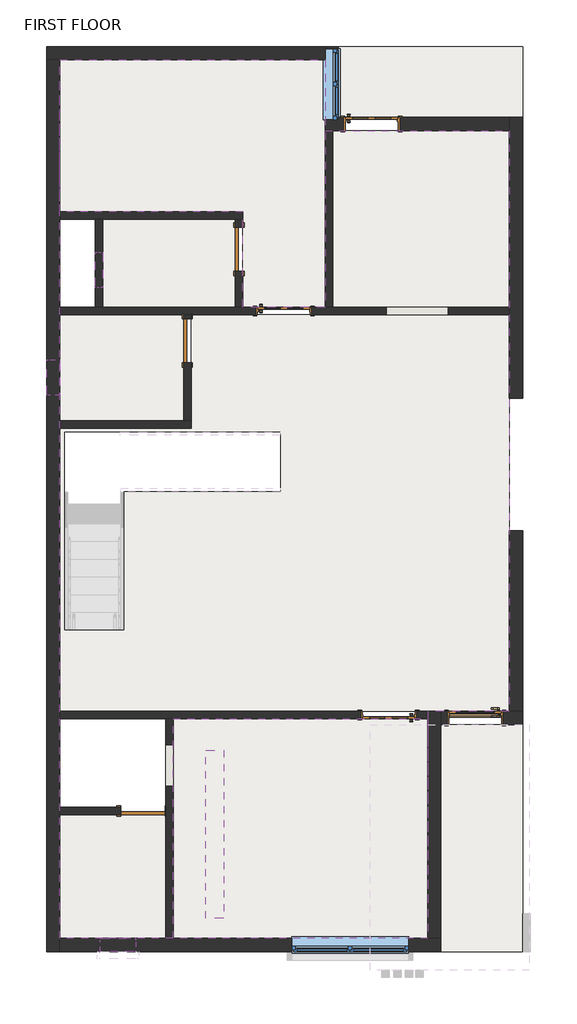
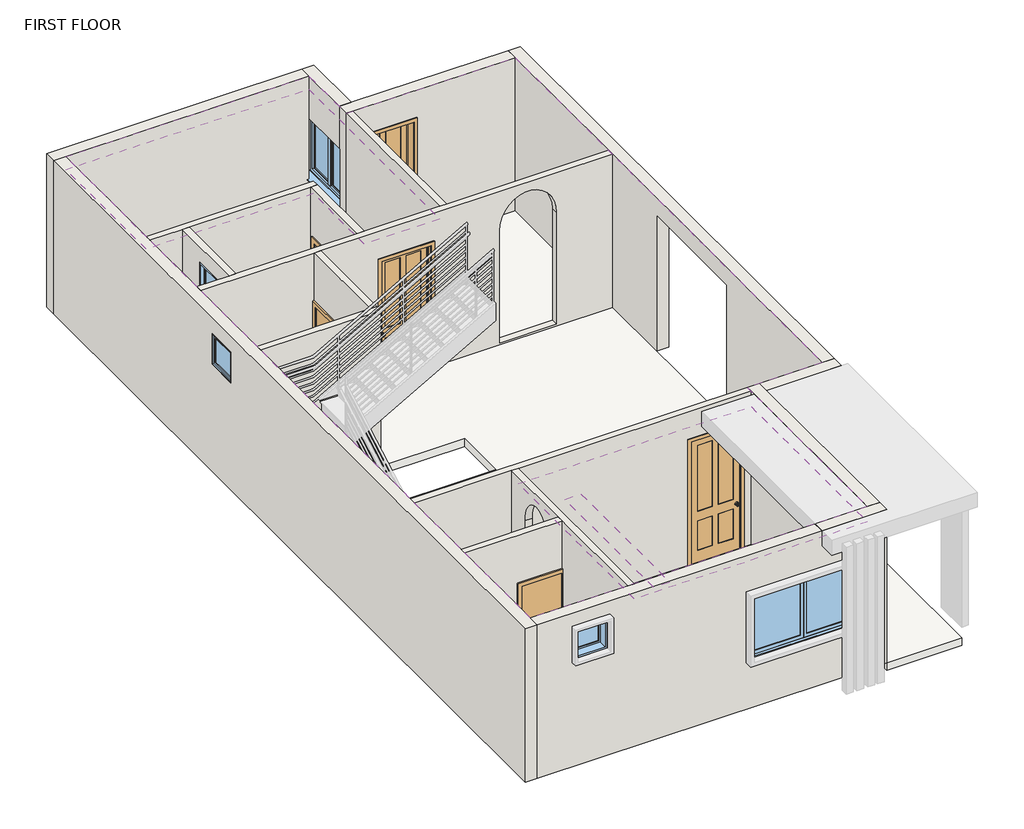
# One storey, part 1 of 3: 18 walls, 7 doors, 5 windows, 3 coverings, 3 slabs, 1 roof.
"""IFC4 building model written with IfcOpenShell, lengths in millimetres."""

from ifc_helpers import new_model, si_unit, point, frame, origin, place, context, project, spatial, polyline, ellipse_curve, trimmed, outline, extrude, faceted_brep, transform, mapped, element, save
from ifc_brep_helpers import plane_surface, extruded_surface, advanced_brep
from components import door_16625766, door_72f69035, door_4f3f9908, door_1fe7f57d, window_80340324, window_d757e824, w2_window_4_x_4_9dec5fc7, w2_window_6_x_4_7b90d420

model = new_model("IFC4")

# Units and contexts
model_context = context("Model", 3, world=origin())
ifc_project = project(units=[si_unit("LENGTHUNIT", "METRE", prefix="MILLI")], contexts=[model_context])

# Site, building, storey
site = spatial("IfcSite", under=ifc_project)
building = spatial("IfcBuilding", under=site)
storey = spatial("IfcBuildingStorey", under=building, Name="FIRST FLOOR", Elevation=3352.8)

# Coverings
placement = place(None, origin())
element("IfcCovering", 1, at=placement, inside=storey, context=model_context, shape_type="SweptSolid", body=[
    extrude(outline(polyline([(-4259.325552, -303.3614843), (-4259.325552, -3198.9614843), (-4564.125552, -3198.9614843), (-4564.125552, -303.3614843), (-4259.325552, -303.3614843)])), frame((0.0, 0.0, 5918.2), z_axis=(0.0, 0.0, 1.0), x_axis=(1.0, 0.0, 0.0)), (0.0, 0.0, 1.0), 41.275),
    extrude(outline(polyline([(-3649.725552, -303.3614843), (-3649.725552, -3198.9614843), (-3954.525552, -3198.9614843), (-3954.525552, -303.3614843), (-3649.725552, -303.3614843)])), frame((0.0, 0.0, 5918.2), z_axis=(0.0, 0.0, 1.0), x_axis=(1.0, 0.0, 0.0)), (0.0, 0.0, 1.0), 41.275),
    extrude(outline(polyline([(-3065.525552, -303.3614843), (-3065.525552, -3198.9614843), (-3370.325552, -3198.9614843), (-3370.325552, -303.3614843), (-3065.525552, -303.3614843)])), frame((0.0, 0.0, 5918.2), z_axis=(0.0, 0.0, 1.0), x_axis=(1.0, 0.0, 0.0)), (0.0, 0.0, 1.0), 41.275),
    extrude(outline(polyline([(-2455.925552, -303.3614843), (-2455.925552, -3198.9614843), (-2760.725552, -3198.9614843), (-2760.725552, -303.3614843), (-2455.925552, -303.3614843)])), frame((0.0, 0.0, 5918.2), z_axis=(0.0, 0.0, 1.0), x_axis=(1.0, 0.0, 0.0)), (0.0, 0.0, 1.0), 41.275),
    extrude(outline(polyline([(-1846.325552, -303.3614843), (-1846.325552, -3198.9614843), (-2151.125552, -3198.9614843), (-2151.125552, -303.3614843), (-1846.325552, -303.3614843)])), frame((0.0, 0.0, 5918.2), z_axis=(0.0, 0.0, 1.0), x_axis=(1.0, 0.0, 0.0)), (0.0, 0.0, 1.0), 41.275),
    extrude(outline(polyline([(-1236.725552, -303.3614843), (-1236.725552, -3198.9614843), (-1541.525552, -3198.9614843), (-1541.525552, -303.3614843), (-1236.725552, -303.3614843)])), frame((0.0, 0.0, 5918.2), z_axis=(0.0, 0.0, 1.0), x_axis=(1.0, 0.0, 0.0)), (0.0, 0.0, 1.0), 41.275),
])
element("IfcCovering", 2, at=placement, inside=storey, context=model_context, shape_type="SweptSolid", body=[
    extrude(outline(polyline([(-7080.273248, 8978.3133697), (-7080.273248, 11594.5133697), (-2508.273248, 11594.5133697), (-2508.273248, 7327.3133697), (-3930.673248, 7327.3133697), (-3930.673248, 8978.3133697), (-7080.273248, 8978.3133697)]), holes=[polyline([(-6775.473248, 11289.7133697), (-6775.473248, 9283.1133697), (-3625.873248, 9283.1133697), (-3625.873248, 7632.1133697), (-2813.073248, 7632.1133697), (-2813.073248, 11289.7133697), (-6775.473248, 11289.7133697)])]), frame((0.0, 0.0, 6146.8), z_axis=(0.0, 0.0, 1.0), x_axis=(1.0, 0.0, 0.0)), (0.0, 0.0, 1.0), 107.95),
    extrude(outline(polyline([(-3422.673248, 10680.1133697), (-3422.673248, 9892.7133697), (-6165.873248, 9892.7133697), (-6165.873248, 10680.1133697), (-3422.673248, 10680.1133697)])), frame((0.0, 0.0, 6146.8), z_axis=(0.0, 0.0, 1.0), x_axis=(1.0, 0.0, 0.0)), (0.0, 0.0, 1.0), 107.95),
])
element("IfcCovering", 3, ObjectType="METAL STUD WHITE CEILING", at=placement, inside=storey, context=model_context, shape_type="SweptSolid", body=[
    extrude(outline(polyline([(-742.973248, 240.7133697), (-742.973248, -3543.8866303), (-5124.473248, -3543.8866303), (-5124.473248, 240.7133697), (-742.973248, 240.7133697)]), holes=[polyline([(-1047.773248, -64.0866303), (-4819.673248, -64.0866303), (-4819.673248, -3239.0866303), (-1047.773248, -3239.0866303), (-1047.773248, -64.0866303)])]), frame((0.0, 0.0, 6096.0), z_axis=(0.0, 0.0, 1.0), x_axis=(1.0, 0.0, 0.0)), (0.0, 0.0, 1.0), 107.95),
])

# Doors
door_shape = door_16625766(model_context)
element("IfcDoor", 4, ObjectType="36\" x 84\"", at=placement, inside=storey, context=model_context, shape_type="MappedRepresentation", body=[
    mapped(door_shape, transform((76.176752, 256.5883697, 3352.8), x_axis=(1.0, 0.0, 0.0), y_axis=(0.0, 1.0, 0.0), z_axis=(0.0, 0.0, 1.0))),
])
door_2_shape = door_72f69035(model_context)
element("IfcDoor", 5, ObjectType="Door-Interior-Single-4_Panel-Wood : 36\" x 96\"", at=placement, inside=storey, context=model_context, shape_type="MappedRepresentation", body=[
    mapped(door_2_shape, transform((-1416.073248, 301.0383697, 3352.8), x_axis=(-1.0, 0.0, 0.0), y_axis=(0.0, -1.0, 0.0), z_axis=(0.0, 0.0, 1.0))),
])
element("IfcDoor", 6, ObjectType="Door-Interior-Single-4_Panel-Wood : 36\" x 96\"", at=placement, inside=storey, context=model_context, shape_type="MappedRepresentation", body=[
    mapped(door_2_shape, transform((-3219.473248, 7266.9883697, 3352.8), x_axis=(1.0, 0.0, 0.0), y_axis=(0.0, 1.0, 0.0), z_axis=(0.0, 0.0, 1.0))),
])
door_3_shape = door_4f3f9908(model_context)
element("IfcDoor", 7, ObjectType="Door-Interior-Single-4_Panel-Wood : 36\" x 96\"", at=placement, inside=storey, context=model_context, shape_type="MappedRepresentation", body=[
    mapped(door_3_shape, transform((-1708.173248, 10492.7883697, 3352.8), x_axis=(1.0, 0.0, 0.0), y_axis=(0.0, 1.0, 0.0), z_axis=(0.0, 0.0, 1.0))),
])
door_4_shape = door_1fe7f57d(model_context)
element("IfcDoor", 8, ObjectType="Single-Flush : 30\" x 80\"", at=placement, inside=storey, context=model_context, shape_type="MappedRepresentation", body=[
    mapped(door_4_shape, transform((-4883.173248, 6755.8133697, 3352.8), x_axis=(0.0, 1.0, 0.0), y_axis=(-1.0, 0.0, 0.0), z_axis=(0.0, 0.0, 1.0))),
])
element("IfcDoor", 9, ObjectType="Single-Flush : 30\" x 80\"", at=placement, inside=storey, context=model_context, shape_type="MappedRepresentation", body=[
    mapped(door_4_shape, transform((-3994.173248, 8330.6133697, 3352.8), x_axis=(0.0, 1.0, 0.0), y_axis=(-1.0, 0.0, 0.0), z_axis=(0.0, 0.0, 1.0))),
])
element("IfcDoor", 10, ObjectType="Single-Flush : 30\" x 80\"", at=placement, inside=storey, context=model_context, shape_type="MappedRepresentation", body=[
    mapped(door_4_shape, transform((-5645.173248, -1346.7866303, 3352.8), x_axis=(-1.0, 0.0, 0.0), y_axis=(0.0, -1.0, 0.0), z_axis=(0.0, 0.0, 1.0))),
])

# Roof
element("IfcRoof", 11, ObjectType="carpet roof 6\"", at=placement, inside=storey, context=model_context, shape_type="SweptSolid", body=[
    extrude(outline(polyline([(-7080.273248, 11594.5133697), (-2508.273248, 11594.5133697), (-2508.273248, 10375.3133697), (666.726752, 10375.3133697), (666.726752, 367.7133697), (-742.973248, 367.7133697), (-742.973248, -3543.8866303), (-7080.273248, -3543.8866303), (-7080.273248, 11594.5133697)]), holes=[polyline([(-3284.0757327, 4159.027543), (-3284.0757327, 5175.027543), (-6992.4757327, 5175.027543), (-6992.4757327, 2787.427543), (-5976.4757327, 2787.427543), (-5976.4757327, 4159.027543), (-3284.0757327, 4159.027543)])]), frame((0.0, 0.0, 6400.8), z_axis=(0.0, 0.0, 1.0), x_axis=(1.0, 0.0, 0.0)), (0.0, 0.0, 1.0), 152.4),
])

# Slabs
element("IfcSlab", 12, at=placement, inside=storey, context=model_context, shape_type="SweptSolid", body=[
    extrude(outline(polyline([(-4057.673248, 8851.3133697), (-4057.673248, 7327.3133697), (-6343.673248, 7327.3133697), (-6343.673248, 8851.3133697), (-4057.673248, 8851.3133697)])), frame((0.0, 0.0, 3200.4), z_axis=(0.0, 0.0, 1.0), x_axis=(1.0, 0.0, 0.0)), (0.0, 0.0, 1.0), 152.4),
    extrude(outline(polyline([(-4946.673248, 7200.3133697), (-4946.673248, 5371.5133697), (-7080.273248, 5371.5133697), (-7080.273248, 7200.3133697), (-4946.673248, 7200.3133697)])), frame((0.0, 0.0, 3200.4), z_axis=(0.0, 0.0, 1.0), x_axis=(1.0, 0.0, 0.0)), (0.0, 0.0, 1.0), 152.4),
    extrude(outline(polyline([(-5264.173248, -3543.8866303), (-7080.273248, -3543.8866303), (-7080.273248, -1410.2866303), (-5264.173248, -1410.2866303), (-5264.173248, -3543.8866303)])), frame((0.0, 0.0, 3200.4), z_axis=(0.0, 0.0, 1.0), x_axis=(1.0, 0.0, 0.0)), (0.0, 0.0, 1.0), 152.4),
])
element("IfcSlab", 13, ObjectType="MARBLE FLOORING 6\"", at=placement, inside=storey, context=model_context, shape_type="SweptSolid", body=[
    extrude(outline(polyline([(666.726752, 10375.3133697), (666.726752, 7327.3133697), (-2381.273248, 7327.3133697), (-2381.273248, 10375.3133697), (666.726752, 10375.3133697)])), frame((0.0, 0.0, 3200.4), z_axis=(0.0, 0.0, 1.0), x_axis=(1.0, 0.0, 0.0)), (0.0, 0.0, 1.0), 152.4),
    extrude(outline(polyline([(-742.973248, 240.7133697), (-742.973248, -3543.8866303), (-5124.473248, -3543.8866303), (-5124.473248, 240.7133697), (-742.973248, 240.7133697)])), frame((0.0, 0.0, 3200.4), z_axis=(0.0, 0.0, 1.0), x_axis=(1.0, 0.0, 0.0)), (0.0, 0.0, 1.0), 152.4),
    extrude(outline(polyline([(-7080.273248, 8978.3133697), (-7080.273248, 11594.5133697), (-2508.273248, 11594.5133697), (-2508.273248, 7327.3133697), (-3930.673248, 7327.3133697), (-3930.673248, 8978.3133697), (-7080.273248, 8978.3133697)])), frame((0.0, 0.0, 3200.4), z_axis=(0.0, 0.0, 1.0), x_axis=(1.0, 0.0, 0.0)), (0.0, 0.0, 1.0), 152.4),
    extrude(outline(polyline([(666.726752, 367.7133697), (-7080.273248, 367.7133697), (-7080.273248, 5244.5133697), (-4819.673248, 5244.5133697), (-4819.673248, 7200.3133697), (666.726752, 7200.3133697), (666.726752, 367.7133697)]), holes=[polyline([(-3284.0757327, 5175.027543), (-6992.4757327, 5175.027543), (-6992.4757327, 1771.427543), (-5976.4757327, 1771.427543), (-5976.4757327, 4159.027543), (-3284.0757327, 4159.027543), (-3284.0757327, 5175.027543)])]), frame((0.0, 0.0, 3200.4), z_axis=(0.0, 0.0, 1.0), x_axis=(1.0, 0.0, 0.0)), (0.0, 0.0, 1.0), 152.4),
])
element("IfcSlab", 14, ObjectType="MARBLE FLOORING 6\"", at=placement, inside=storey, context=model_context, shape_type="SweptSolid", body=[
    extrude(outline(polyline([(895.326752, 139.1133697), (895.326752, -3772.4866303), (-514.373248, -3772.4866303), (-514.373248, 139.1133697), (895.326752, 139.1133697)])), frame((0.0, 0.0, 3200.4), z_axis=(0.0, 0.0, 1.0), x_axis=(1.0, 0.0, 0.0)), (0.0, 0.0, 1.0), 152.4),
    extrude(outline(polyline([(895.326752, 10603.9133697), (-2279.673248, 10603.9133697), (-2279.673248, 11823.1133697), (895.326752, 11823.1133697), (895.326752, 10603.9133697)])), frame((0.0, 0.0, 3200.4), z_axis=(0.0, 0.0, 1.0), x_axis=(1.0, 0.0, 0.0)), (0.0, 0.0, 1.0), 152.4),
])

# Walls
element("IfcWall", 15, ObjectType="INNER WALL 5\"", at=placement, inside=storey, context=model_context, shape_type="AdvancedBrep", body=[
    advanced_brep(
    [(-5124.473248, -3543.8866303, 3352.8), (-5124.473248, 240.7133697, 3352.8), (-5124.473248, 240.7133697, 6400.8), (-5124.473248, -3543.8866303, 6400.8), (-5124.473248, -211.107669, 3493.0989834), (-5124.473248, -921.3329942, 3493.0989834), (-5124.473248, -921.3329942, 5715.1596494), (-5124.473248, -211.107669, 5677.9383173), (-5251.473248, -3543.8866303, 3352.8), (-5251.473248, -3543.8866303, 6400.8), (-5251.473248, -1410.2866303, 6400.8), (-5251.473248, -1283.2866303, 6400.8), (-5251.473248, 240.7133697, 6400.8), (-5251.473248, 240.7133697, 3352.8), (-5251.473248, -1283.2866303, 3352.8), (-5251.473248, -1410.2866303, 3352.8), (-5251.473248, -211.107669, 3493.0989834), (-5251.473248, -211.107669, 5677.9383173), (-5251.473248, -921.3329942, 5715.1596494), (-5251.473248, -921.3329942, 3493.0989834)],
    [
        (0, 1),
        (1, 2),
        (2, 3),
        (3, 0),
        (4, 5),
        (5, 6),
        (6, 7, ellipse_curve(frame((-5124.473248, -566.2203316, 5696.5489834), z_axis=(-0.9999999999999999, 0.0, 0.0), x_axis=(0.0, -0.05233595624293513, -0.9986295347545743)), 457.2, 355.6)),
        (7, 4),
        (8, 9),
        (9, 10),
        (10, 11),
        (11, 12),
        (12, 13),
        (13, 14),
        (14, 15),
        (15, 8),
        (16, 17),
        (17, 18, ellipse_curve(frame((-5251.473248, -566.2203316, 5696.5489834), z_axis=(0.9999999999999999, 0.0, 0.0), x_axis=(0.0, -0.05233595624293513, -0.9986295347545743)), 457.2, 355.6)),
        (18, 19),
        (19, 16),
        (3, 9),
        (8, 0),
        (1, 13),
        (12, 2),
        (4, 16),
        (19, 5),
        (18, 6),
        (17, 7),
    ],
    [
        plane_surface(frame((-5124.473248, -3658.1866303, 3352.8), z_axis=(1.0, 0.0, 0.0), x_axis=(0.0, 1.0, 0.0))),
        plane_surface(frame((-5251.473248, -3658.1866303, 3352.8), z_axis=(-1.0, 0.0, 0.0), x_axis=(0.0, -1.0, 0.0))),
        plane_surface(frame((-7219.973248, -3543.8866303, 3352.8), z_axis=(0.0, -1.0, 0.0), x_axis=(-1.0, 0.0, 0.0))),
        plane_surface(frame((-742.973248, 240.7133697, 3352.8), z_axis=(0.0, 1.0, 0.0), x_axis=(1.0, 0.0, 0.0))),
        plane_surface(frame((-5124.473248, -3658.1866303, 3352.8), z_axis=(0.0, 0.0, -1.0), x_axis=(-1.0, 0.0, 0.0))),
        plane_surface(frame((-5124.473248, 304.2133697, 6400.8), z_axis=(0.0, 0.0, 1.0), x_axis=(-1.0, 0.0, 0.0))),
        plane_surface(frame((-5124.473248, -211.107669, 3493.0989834), z_axis=(0.0, 0.0, 1.0), x_axis=(-1.0, 0.0, 0.0))),
        plane_surface(frame((-5124.473248, -921.3329942, 3493.0989834), z_axis=(0.0, 1.0, 0.0), x_axis=(-1.0, 0.0, 0.0))),
        extruded_surface(trimmed(ellipse_curve(frame((-5314.973248, -566.2203316, 5696.5489834), z_axis=(-0.9999999999999999, 0.0, 0.0), x_axis=(0.0, 0.9986295347545743, -0.05233595624293513)), 355.6, 457.2), [point((-5314.973248, -921.3329942, 5715.1596494))], [point((-5314.973248, -211.107669, 5677.9383173))], True, "CARTESIAN"), (127.0, 0.0, 0.0), 127.0),
        plane_surface(frame((-5124.473248, -211.107669, 5677.9383173), z_axis=(0.0, -1.0, 0.0), x_axis=(-1.0, 0.0, 0.0))),
    ],
    [
        (0, [[1, 2, 3, 4], [5, 6, 7, 8]]),
        (1, [[9, 10, 11, 12, 13, 14, 15, 16], [17, 18, 19, 20]]),
        (2, [[-4, 21, -9, 22]]),
        (3, [[-2, 23, -13, 24]]),
        (4, [[-1, -22, -16, -15, -14, -23]]),
        (5, [[-3, -24, -12, -11, -10, -21]]),
        (6, [[-5, 25, -20, 26]]),
        (7, [[-6, -26, -19, 27]]),
        (8, [[-7, -27, -18, 28]]),
        (9, [[-8, -28, -17, -25]]),
    ],
),
])
element("IfcWall", 16, ObjectType="INNER WALL 5\"", at=placement, inside=storey, context=model_context, shape_type="SweptSolid", body=[
    extrude(outline(polyline([(3352.8, -7080.273248), (3352.8, -6026.173248), (5384.8, -6026.173248), (5384.8, -5264.173248), (3352.8, -5264.173248), (3352.8, -5251.473248), (6400.8, -5251.473248), (6400.8, -7080.273248), (3352.8, -7080.273248)])), frame((0.0, -1410.2866303, 0.0), z_axis=(0.0, 1.0, 0.0), x_axis=(0.0, 0.0, 1.0)), (0.0, 0.0, 1.0), 127.0),
])
element("IfcWall", 17, ObjectType="INNER WALL 5\"", at=placement, inside=storey, context=model_context, shape_type="Brep", body=[
    faceted_brep([(-7080.273248, 367.7133697, 6400.8), (-742.973248, 367.7133697, 6400.8), (-742.973248, 367.7133697, 3352.8), (-933.473248, 367.7133697, 3352.8), (-933.473248, 367.7133697, 5816.6), (-1898.673248, 367.7133697, 5816.6), (-1898.673248, 367.7133697, 3352.8), (-7080.273248, 367.7133697, 3352.8), (-742.973248, 240.7133697, 6400.8), (-5124.473248, 240.7133697, 6400.8), (-5251.473248, 240.7133697, 6400.8), (-7080.273248, 240.7133697, 6400.8), (-7080.273248, 240.7133697, 3352.8), (-5251.473248, 240.7133697, 3352.8), (-5124.473248, 240.7133697, 3352.8), (-1898.673248, 240.7133697, 3352.8), (-1898.673248, 240.7133697, 5816.6), (-933.473248, 240.7133697, 5816.6), (-933.473248, 240.7133697, 3352.8), (-742.973248, 240.7133697, 3352.8)], [[[0, 1, 2, 3, 4, 5, 6, 7]], [[8, 9, 10, 11, 12, 13, 14, 15, 16, 17, 18, 19]], [[2, 19, 18, 3]], [[12, 7, 6, 15, 14, 13]], [[1, 0, 11, 10, 9, 8]], [[2, 1, 8, 19]], [[0, 7, 12, 11]], [[5, 16, 15, 6]], [[16, 5, 4, 17]], [[17, 4, 3, 18]]]),
])
element("IfcWall", 18, ObjectType="INNER WALL 5\"", at=placement, inside=storey, context=model_context, shape_type="AdvancedBrep", body=[
    advanced_brep(
    [(666.726752, 7200.3133697, 6400.8), (-4819.673248, 7200.3133697, 6400.8), (-4946.673248, 7200.3133697, 6400.8), (-7080.273248, 7200.3133697, 6400.8), (-7080.273248, 7200.3133697, 3352.8), (-4946.673248, 7200.3133697, 3352.8), (-4819.673248, 7200.3133697, 3352.8), (-3702.073248, 7200.3133697, 3352.8), (-3702.073248, 7200.3133697, 5816.6), (-2736.873248, 7200.3133697, 5816.6), (-2736.873248, 7200.3133697, 3352.8), (666.726752, 7200.3133697, 3352.8), (-387.8615631, 7200.3133697, 3392.0138877), (-1454.6615631, 7200.3133697, 3392.0138877), (-1454.6615631, 7200.3133697, 5366.5977751), (-1454.6615631, 7200.3133697, 5614.5138877), (-387.8615631, 7200.3133697, 5614.5138877), (-7080.273248, 7327.3133697, 6400.8), (-6470.673248, 7327.3133697, 6400.8), (-6343.673248, 7327.3133697, 6400.8), (-4057.673248, 7327.3133697, 6400.8), (-3930.673248, 7327.3133697, 6400.8), (-2508.273248, 7327.3133697, 6400.8), (-2381.273248, 7327.3133697, 6400.8), (666.726752, 7327.3133697, 6400.8), (666.726752, 7327.3133697, 3352.8), (-2381.273248, 7327.3133697, 3352.8), (-2508.273248, 7327.3133697, 3352.8), (-2736.873248, 7327.3133697, 3352.8), (-2736.873248, 7327.3133697, 5816.6), (-3702.073248, 7327.3133697, 5816.6), (-3702.073248, 7327.3133697, 3352.8), (-3930.673248, 7327.3133697, 3352.8), (-4057.673248, 7327.3133697, 3352.8), (-6343.673248, 7327.3133697, 3352.8), (-6470.673248, 7327.3133697, 3352.8), (-7080.273248, 7327.3133697, 3352.8), (-1454.6615631, 7327.3133697, 3392.0138877), (-387.8615631, 7327.3133697, 3392.0138877), (-387.8615631, 7327.3133697, 5614.5138877), (-1454.6615631, 7327.3133697, 5614.5138877), (-1454.6615631, 7327.3133697, 5366.5977751)],
    [
        (0, 1),
        (1, 2),
        (2, 3),
        (3, 4),
        (4, 5),
        (5, 6),
        (6, 7),
        (7, 8),
        (8, 9),
        (9, 10),
        (10, 11),
        (11, 0),
        (12, 13),
        (13, 14),
        (14, 15),
        (15, 16, ellipse_curve(frame((-921.2615631, 7200.3133697, 5614.5138877), z_axis=(0.0, 1.0, 0.0), x_axis=(0.0, 0.0, -1.0)), 609.6, 533.4)),
        (16, 12),
        (17, 18),
        (18, 19),
        (19, 20),
        (20, 21),
        (21, 22),
        (22, 23),
        (23, 24),
        (24, 25),
        (25, 26),
        (26, 27),
        (27, 28),
        (28, 29),
        (29, 30),
        (30, 31),
        (31, 32),
        (32, 33),
        (33, 34),
        (34, 35),
        (35, 36),
        (36, 17),
        (37, 38),
        (38, 39),
        (39, 40, ellipse_curve(frame((-921.2615631, 7327.3133697, 5614.5138877), z_axis=(0.0, -1.0, 0.0), x_axis=(0.0, 0.0, -1.0)), 609.6, 533.4)),
        (40, 41),
        (41, 37),
        (3, 17),
        (36, 4),
        (11, 25),
        (24, 0),
        (31, 7),
        (10, 28),
        (12, 38),
        (37, 13),
        (41, 14),
        (40, 15),
        (39, 16),
        (9, 29),
        (8, 30),
    ],
    [
        plane_surface(frame((-7194.573248, 7200.3133697, 3352.8), z_axis=(0.0, -1.0, 0.0), x_axis=(1.0, 0.0, 0.0))),
        plane_surface(frame((-7194.573248, 7327.3133697, 3352.8), z_axis=(0.0, 1.0, 0.0), x_axis=(-1.0, 0.0, 0.0))),
        plane_surface(frame((-7080.273248, 8571.9133697, 3352.8), z_axis=(-1.0, 0.0, 0.0), x_axis=(0.0, 1.0, 0.0))),
        plane_surface(frame((666.726752, 1256.7133697, 3352.8), z_axis=(1.0, 0.0, 0.0), x_axis=(0.0, -1.0, 0.0))),
        plane_surface(frame((-7194.573248, 7200.3133697, 3352.8), z_axis=(0.0, 0.0, -1.0), x_axis=(0.0, 1.0, 0.0))),
        plane_surface(frame((781.026752, 7200.3133697, 6400.8), z_axis=(0.0, 0.0, 1.0), x_axis=(0.0, 1.0, 0.0))),
        plane_surface(frame((-387.8615631, 7200.3133697, 3392.0138877), z_axis=(0.0, 0.0, 1.0), x_axis=(0.0, 1.0, 0.0))),
        plane_surface(frame((-1454.6615631, 7200.3133697, 3392.0138877), z_axis=(1.0, 0.0, 0.0), x_axis=(0.0, 1.0, 0.0))),
        plane_surface(frame((-1454.6615631, 7200.3133697, 5366.5977751), z_axis=(1.0, 0.0, 0.0), x_axis=(0.0, 1.0, 0.0))),
        extruded_surface(trimmed(ellipse_curve(frame((-921.2615631, 7390.8133697, 5614.5138877), z_axis=(0.0, 1.0, 0.0), x_axis=(1.0, 0.0, 0.0)), 533.4, 609.6), [point((-1454.6615631, 7390.8133697, 5614.5138877))], [point((-387.8615631, 7390.8133697, 5614.5138877))], True, "CARTESIAN"), (0.0, -127.0, 0.0), 127.0),
        plane_surface(frame((-387.8615631, 7200.3133697, 5614.5138877), z_axis=(-1.0, 0.0, 0.0), x_axis=(0.0, 1.0, 0.0))),
        plane_surface(frame((-2736.873248, 5676.3133697, 3352.8), z_axis=(-1.0, 0.0, 0.0), x_axis=(0.0, 1.0, 0.0))),
        plane_surface(frame((-2736.873248, 5676.3133697, 5816.6), z_axis=(0.0, 0.0, -1.0), x_axis=(0.0, 1.0, 0.0))),
        plane_surface(frame((-3702.073248, 5676.3133697, 5816.6), z_axis=(1.0, 0.0, 0.0), x_axis=(0.0, 1.0, 0.0))),
    ],
    [
        (0, [[1, 2, 3, 4, 5, 6, 7, 8, 9, 10, 11, 12], [13, 14, 15, 16, 17]]),
        (1, [[18, 19, 20, 21, 22, 23, 24, 25, 26, 27, 28, 29, 30, 31, 32, 33, 34, 35, 36, 37], [38, 39, 40, 41, 42]]),
        (2, [[-4, 43, -37, 44]]),
        (3, [[-12, 45, -25, 46]]),
        (4, [[-44, -36, -35, -34, -33, -32, 47, -7, -6, -5]]),
        (4, [[-45, -11, 48, -28, -27, -26]]),
        (5, [[-3, -2, -1, -46, -24, -23, -22, -21, -20, -19, -18, -43]]),
        (6, [[-13, 49, -38, 50]]),
        (7, [[-14, -50, -42, 51]]),
        (8, [[-15, -51, -41, 52]]),
        (9, [[-16, -52, -40, 53]]),
        (10, [[-17, -53, -39, -49]]),
        (11, [[54, -29, -48, -10]]),
        (12, [[-54, -9, 55, -30]]),
        (13, [[-55, -8, -47, -31]]),
    ],
),
])
element("IfcWall", 19, ObjectType="INNER WALL 5\"", at=placement, inside=storey, context=model_context, shape_type="SweptSolid", body=[
    extrude(outline(polyline([(-2508.273248, 7327.3133697), (-2508.273248, 10375.3133697), (-2381.273248, 10375.3133697), (-2381.273248, 7327.3133697), (-2508.273248, 7327.3133697)])), frame((0.0, 0.0, 3352.8), z_axis=(0.0, 0.0, 1.0), x_axis=(1.0, 0.0, 0.0)), (0.0, 0.0, 1.0), 3048.0),
])
element("IfcWall", 20, ObjectType="INNER WALL 5\"", at=placement, inside=storey, context=model_context, shape_type="Brep", body=[
    faceted_brep([(-7080.273248, 5244.5133697, 3352.8), (-4819.673248, 5244.5133697, 3352.8), (-4819.673248, 5244.5133697, 6400.8), (-7080.273248, 5244.5133697, 6400.8), (-7080.273248, 5371.5133697, 3352.8), (-7080.273248, 5371.5133697, 6400.8), (-4946.673248, 5371.5133697, 6400.8), (-4819.673248, 5371.5133697, 6400.8), (-4819.673248, 5371.5133697, 3352.8), (-4946.673248, 5371.5133697, 3352.8)], [[[0, 1, 2, 3]], [[4, 5, 6, 7, 8, 9]], [[1, 0, 4, 9, 8]], [[3, 2, 7, 6, 5]], [[0, 3, 5, 4]], [[2, 1, 8, 7]]]),
])
element("IfcWall", 21, ObjectType="INNER WALL 5\"", at=placement, inside=storey, context=model_context, shape_type="SweptSolid", body=[
    extrude(outline(polyline([(7200.3133697, 3352.8), (7136.8133697, 3352.8), (7136.8133697, 5384.8), (6374.8133697, 5384.8), (6374.8133697, 3352.8), (5371.5133697, 3352.8), (5371.5133697, 6400.8), (7200.3133697, 6400.8), (7200.3133697, 3352.8)])), frame((-4946.673248, 0.0, 0.0), z_axis=(1.0, 0.0, 0.0), x_axis=(0.0, 1.0, 0.0)), (0.0, 0.0, 1.0), 127.0),
])
element("IfcWall", 22, ObjectType="INNER WALL 5\"", at=placement, inside=storey, context=model_context, shape_type="Brep", body=[
    faceted_brep([(-7080.273248, 8851.3133697, 3352.8), (-6470.673248, 8851.3133697, 3352.8), (-6343.673248, 8851.3133697, 3352.8), (-4057.673248, 8851.3133697, 3352.8), (-3930.673248, 8851.3133697, 3352.8), (-3930.673248, 8851.3133697, 6400.8), (-4057.673248, 8851.3133697, 6400.8), (-6343.673248, 8851.3133697, 6400.8), (-6470.673248, 8851.3133697, 6400.8), (-7080.273248, 8851.3133697, 6400.8), (-7080.273248, 8978.3133697, 3352.8), (-7080.273248, 8978.3133697, 6400.8), (-3930.673248, 8978.3133697, 6400.8), (-3930.673248, 8978.3133697, 3352.8)], [[[0, 1, 2, 3, 4, 5, 6, 7, 8, 9]], [[10, 11, 12, 13]], [[4, 3, 2, 1, 0, 10, 13]], [[9, 8, 7, 6, 5, 12, 11]], [[0, 9, 11, 10]], [[5, 4, 13, 12]]]),
])
element("IfcWall", 23, ObjectType="INNER WALL 5\"", at=placement, inside=storey, context=model_context, shape_type="SweptSolid", body=[
    extrude(outline(polyline([(7327.3133697, 6400.8), (8851.3133697, 6400.8), (8851.3133697, 3352.8), (8711.6133697, 3352.8), (8711.6133697, 5384.8), (7949.6133697, 5384.8), (7949.6133697, 3352.8), (7327.3133697, 3352.8), (7327.3133697, 6400.8)])), frame((-4057.673248, 0.0, 0.0), z_axis=(1.0, 0.0, 0.0), x_axis=(0.0, 1.0, 0.0)), (0.0, 0.0, 1.0), 127.0),
])
element("IfcWall", 24, ObjectType="INNER WALL 5\"", at=placement, inside=storey, context=model_context, shape_type="SweptSolid", body=[
    extrude(outline(polyline([(8851.3133697, 3352.8), (7327.3133697, 3352.8), (7327.3133697, 6400.8), (8851.3133697, 6400.8), (8851.3133697, 3352.8)]), holes=[polyline([(7670.2133697, 6096.0), (7670.2133697, 5486.4), (8279.8133697, 5486.4), (8279.8133697, 6096.0), (7670.2133697, 6096.0)])]), frame((-6470.673248, 0.0, 0.0), z_axis=(1.0, 0.0, 0.0), x_axis=(0.0, 1.0, 0.0)), (0.0, 0.0, 1.0), 127.0),
])
element("IfcWall", 25, ObjectType="OUTER WALL 9\"", at=placement, inside=storey, context=model_context, shape_type="Brep", body=[
    faceted_brep([(-7308.873248, 11594.5133697, 3352.8), (-7308.873248, -3772.4866303, 3352.8), (-7308.873248, -3772.4866303, 6400.8), (-7308.873248, 11594.5133697, 6400.8), (-7308.873248, 6425.6133697, 6096.0), (-7308.873248, 5816.0133697, 6096.0), (-7308.873248, 5816.0133697, 5486.4), (-7308.873248, 6425.6133697, 5486.4), (-7080.273248, 11594.5133697, 3352.8), (-7080.273248, 11594.5133697, 6400.8), (-7080.273248, 8978.3133697, 6400.8), (-7080.273248, 8851.3133697, 6400.8), (-7080.273248, 7327.3133697, 6400.8), (-7080.273248, 7200.3133697, 6400.8), (-7080.273248, 5371.5133697, 6400.8), (-7080.273248, 5244.5133697, 6400.8), (-7080.273248, 367.7133697, 6400.8), (-7080.273248, 240.7133697, 6400.8), (-7080.273248, -1283.2866303, 6400.8), (-7080.273248, -1410.2866303, 6400.8), (-7080.273248, -3543.8866303, 6400.8), (-7080.273248, -3772.4866303, 6400.8), (-7080.273248, -3772.4866303, 3352.8), (-7080.273248, -3543.8866303, 3352.8), (-7080.273248, -1410.2866303, 3352.8), (-7080.273248, -1283.2866303, 3352.8), (-7080.273248, 240.7133697, 3352.8), (-7080.273248, 367.7133697, 3352.8), (-7080.273248, 5244.5133697, 3352.8), (-7080.273248, 5371.5133697, 3352.8), (-7080.273248, 7200.3133697, 3352.8), (-7080.273248, 7327.3133697, 3352.8), (-7080.273248, 8851.3133697, 3352.8), (-7080.273248, 8978.3133697, 3352.8), (-7080.273248, 6425.6133697, 6096.0), (-7080.273248, 6425.6133697, 5486.4), (-7080.273248, 5816.0133697, 5486.4), (-7080.273248, 5816.0133697, 6096.0)], [[[0, 1, 2, 3], [4, 5, 6, 7]], [[8, 9, 10, 11, 12, 13, 14, 15, 16, 17, 18, 19, 20, 21, 22, 23, 24, 25, 26, 27, 28, 29, 30, 31, 32, 33], [34, 35, 36, 37]], [[1, 0, 8, 33, 32, 31, 30, 29, 28, 27, 26, 25, 24, 23, 22]], [[3, 2, 21, 20, 19, 18, 17, 16, 15, 14, 13, 12, 11, 10, 9]], [[2, 1, 22, 21]], [[0, 3, 9, 8]], [[35, 34, 4, 7]], [[36, 35, 7, 6]], [[37, 36, 6, 5]], [[34, 37, 5, 4]]]),
])
element("IfcWall", 26, ObjectType="OUTER WALL 9\"", at=placement, inside=storey, context=model_context, shape_type="Brep", body=[
    faceted_brep([(-7080.273248, -3772.4866303, 3352.8), (-514.373248, -3772.4866303, 3352.8), (-514.373248, -3772.4866303, 6400.8), (-7080.273248, -3772.4866303, 6400.8), (-3081.473248, -3772.4866303, 4352.8), (-3081.473248, -3772.4866303, 5612.8), (-1071.473248, -3772.4866303, 5612.8), (-1071.473248, -3772.4866303, 4352.8), (-5772.173248, -3772.4866303, 6096.0), (-5772.173248, -3772.4866303, 5486.4), (-6381.773248, -3772.4866303, 5486.4), (-6381.773248, -3772.4866303, 6096.0), (-7080.273248, -3543.8866303, 3352.8), (-7080.273248, -3543.8866303, 6400.8), (-5251.473248, -3543.8866303, 6400.8), (-5124.473248, -3543.8866303, 6400.8), (-742.973248, -3543.8866303, 6400.8), (-514.373248, -3543.8866303, 6400.8), (-514.373248, -3543.8866303, 3352.8), (-742.973248, -3543.8866303, 3352.8), (-5124.473248, -3543.8866303, 3352.8), (-5251.473248, -3543.8866303, 3352.8), (-3081.473248, -3543.8866303, 4352.8), (-1071.473248, -3543.8866303, 4352.8), (-1071.473248, -3543.8866303, 5612.8), (-3081.473248, -3543.8866303, 5612.8), (-5772.173248, -3543.8866303, 6096.0), (-6381.773248, -3543.8866303, 6096.0), (-6381.773248, -3543.8866303, 5486.4), (-5772.173248, -3543.8866303, 5486.4)], [[[0, 1, 2, 3], [4, 5, 6, 7], [8, 9, 10, 11]], [[12, 13, 14, 15, 16, 17, 18, 19, 20, 21], [22, 23, 24, 25], [26, 27, 28, 29]], [[1, 0, 12, 21, 20, 19, 18]], [[3, 2, 17, 16, 15, 14, 13]], [[0, 3, 13, 12]], [[2, 1, 18, 17]], [[5, 4, 22, 25]], [[6, 5, 25, 24]], [[7, 6, 24, 23]], [[4, 7, 23, 22]], [[9, 8, 26, 29]], [[10, 9, 29, 28]], [[11, 10, 28, 27]], [[8, 11, 27, 26]]]),
])
element("IfcWall", 27, ObjectType="OUTER WALL 9\"", at=placement, inside=storey, context=model_context, shape_type="Brep", body=[
    faceted_brep([(-514.373248, -3543.8866303, 3352.8), (-514.373248, 139.1133697, 3352.8), (-514.373248, 367.7133697, 3352.8), (-514.373248, 367.7133697, 6400.8), (-514.373248, 139.1133697, 6400.8), (-514.373248, -3543.8866303, 6400.8), (-742.973248, -3543.8866303, 3352.8), (-742.973248, -3543.8866303, 6400.8), (-742.973248, 240.7133697, 6400.8), (-742.973248, 367.7133697, 6400.8), (-742.973248, 367.7133697, 3352.8), (-742.973248, 240.7133697, 3352.8)], [[[0, 1, 2, 3, 4, 5]], [[6, 7, 8, 9, 10, 11]], [[2, 1, 0, 6, 11, 10]], [[5, 4, 3, 9, 8, 7]], [[0, 5, 7, 6]], [[3, 2, 10, 9]]]),
])
element("IfcWall", 28, ObjectType="OUTER WALL 9\"", at=placement, inside=storey, context=model_context, shape_type="Brep", body=[
    faceted_brep([(895.326752, 139.1133697, 6400.8), (-514.373248, 139.1133697, 6400.8), (-514.373248, 139.1133697, 3352.8), (-406.423248, 139.1133697, 3352.8), (-406.423248, 139.1133697, 5511.8), (558.776752, 139.1133697, 5511.8), (558.776752, 139.1133697, 3352.8), (895.326752, 139.1133697, 3352.8), (-514.373248, 367.7133697, 6400.8), (666.726752, 367.7133697, 6400.8), (895.326752, 367.7133697, 6400.8), (895.326752, 367.7133697, 3352.8), (666.726752, 367.7133697, 3352.8), (558.776752, 367.7133697, 3352.8), (558.776752, 367.7133697, 5511.8), (-406.423248, 367.7133697, 5511.8), (-406.423248, 367.7133697, 3352.8), (-514.373248, 367.7133697, 3352.8)], [[[0, 1, 2, 3, 4, 5, 6, 7]], [[8, 9, 10, 11, 12, 13, 14, 15, 16, 17]], [[2, 17, 16, 3]], [[11, 7, 6, 13, 12]], [[1, 0, 10, 9, 8]], [[2, 1, 8, 17]], [[0, 7, 11, 10]], [[5, 14, 13, 6]], [[14, 5, 4, 15]], [[15, 4, 3, 16]]]),
])
element("IfcWall", 29, ObjectType="OUTER WALL 9\"", at=placement, inside=storey, context=model_context, shape_type="Brep", body=[
    faceted_brep([(895.326752, 10603.9133697, 6400.8), (895.326752, 367.7133697, 6400.8), (895.326752, 367.7133697, 3352.8), (895.326752, 3479.2133697, 3352.8), (895.326752, 3479.2133697, 6059.5090117), (895.326752, 5765.2133697, 6059.5090117), (895.326752, 5765.2133697, 3352.8), (895.326752, 10603.9133697, 3352.8), (666.726752, 367.7133697, 6400.8), (666.726752, 7200.3133697, 6400.8), (666.726752, 7327.3133697, 6400.8), (666.726752, 10375.3133697, 6400.8), (666.726752, 10603.9133697, 6400.8), (666.726752, 10603.9133697, 3352.8), (666.726752, 10375.3133697, 3352.8), (666.726752, 7327.3133697, 3352.8), (666.726752, 7200.3133697, 3352.8), (666.726752, 5765.2133697, 3352.8), (666.726752, 5765.2133697, 6059.5090117), (666.726752, 3479.2133697, 6059.5090117), (666.726752, 3479.2133697, 3352.8), (666.726752, 367.7133697, 3352.8)], [[[0, 1, 2, 3, 4, 5, 6, 7]], [[8, 9, 10, 11, 12, 13, 14, 15, 16, 17, 18, 19, 20, 21]], [[2, 21, 20, 3]], [[13, 7, 6, 17, 16, 15, 14]], [[1, 0, 12, 11, 10, 9, 8]], [[2, 1, 8, 21]], [[0, 7, 13, 12]], [[19, 4, 3, 20]], [[4, 19, 18, 5]], [[5, 18, 17, 6]]]),
])
element("IfcWall", 30, ObjectType="OUTER WALL 9\"", at=placement, inside=storey, context=model_context, shape_type="Brep", body=[
    faceted_brep([(-2508.273248, 10603.9133697, 6400.8), (-2279.673248, 10603.9133697, 6400.8), (666.726752, 10603.9133697, 6400.8), (666.726752, 10603.9133697, 3352.8), (-1225.573248, 10603.9133697, 3352.8), (-1225.573248, 10603.9133697, 5816.6), (-2190.773248, 10603.9133697, 5816.6), (-2190.773248, 10603.9133697, 3352.8), (-2279.673248, 10603.9133697, 3352.8), (-2508.273248, 10603.9133697, 3352.8), (-2508.273248, 10603.9133697, 4352.8), (-2279.673248, 10603.9133697, 4352.8), (-2279.673248, 10603.9133697, 5572.0), (-2508.273248, 10603.9133697, 5572.0), (666.726752, 10375.3133697, 6400.8), (-2381.273248, 10375.3133697, 6400.8), (-2508.273248, 10375.3133697, 6400.8), (-2508.273248, 10375.3133697, 3352.8), (-2381.273248, 10375.3133697, 3352.8), (-2190.773248, 10375.3133697, 3352.8), (-2190.773248, 10375.3133697, 5816.6), (-1225.573248, 10375.3133697, 5816.6), (-1225.573248, 10375.3133697, 3352.8), (666.726752, 10375.3133697, 3352.8), (-2508.273248, 10565.8133697, 5572.0), (-2508.273248, 10565.8133697, 4352.8), (-2279.673248, 10565.8133697, 4352.8), (-2279.673248, 10565.8133697, 5572.0)], [[[0, 1, 2, 3, 4, 5, 6, 7, 8, 9, 10, 11, 12, 13]], [[14, 15, 16, 17, 18, 19, 20, 21, 22, 23]], [[3, 23, 22, 4]], [[17, 9, 8, 7, 19, 18]], [[2, 1, 0, 16, 15, 14]], [[3, 2, 14, 23]], [[9, 17, 16, 0, 13, 24, 25, 10]], [[26, 27, 12, 11]], [[27, 26, 25, 24]], [[27, 24, 13, 12]], [[25, 26, 11, 10]], [[21, 5, 4, 22]], [[5, 21, 20, 6]], [[6, 20, 19, 7]]]),
])
element("IfcWall", 31, ObjectType="OUTER WALL 9\"", at=placement, inside=storey, context=model_context, shape_type="Brep", body=[
    faceted_brep([(-2279.673248, 10603.9133697, 3352.8), (-2279.673248, 11823.1133697, 3352.8), (-2279.673248, 11823.1133697, 6400.8), (-2279.673248, 10603.9133697, 6400.8), (-2279.673248, 10603.9133697, 5572.0), (-2279.673248, 11785.0133697, 5572.0), (-2279.673248, 11785.0133697, 4352.8), (-2279.673248, 10603.9133697, 4352.8), (-2508.273248, 11823.1133697, 3352.8), (-2508.273248, 11594.5133697, 3352.8), (-2508.273248, 10603.9133697, 3352.8), (-2508.273248, 10603.9133697, 4352.8), (-2508.273248, 11785.0133697, 4352.8), (-2508.273248, 11785.0133697, 5572.0), (-2508.273248, 10603.9133697, 5572.0), (-2508.273248, 10603.9133697, 6400.8), (-2508.273248, 11594.5133697, 6400.8), (-2508.273248, 11823.1133697, 6400.8)], [[[0, 1, 2, 3, 4, 5, 6, 7]], [[8, 9, 10, 11, 12, 13, 14, 15, 16, 17]], [[1, 0, 10, 9, 8]], [[3, 2, 17, 16, 15]], [[3, 15, 14, 4]], [[10, 0, 7, 11]], [[2, 1, 8, 17]], [[13, 5, 4, 14]], [[5, 13, 12, 6]], [[6, 12, 11, 7]]]),
])
element("IfcWall", 32, ObjectType="OUTER WALL 9\"", at=placement, inside=storey, context=model_context, shape_type="Brep", body=[
    faceted_brep([(-2508.273248, 11823.1133697, 3352.8), (-7308.873248, 11823.1133697, 3352.8), (-7308.873248, 11823.1133697, 6400.8), (-2508.273248, 11823.1133697, 6400.8), (-2508.273248, 11594.5133697, 3352.8), (-2508.273248, 11594.5133697, 6400.8), (-7080.273248, 11594.5133697, 6400.8), (-7308.873248, 11594.5133697, 6400.8), (-7308.873248, 11594.5133697, 3352.8), (-7080.273248, 11594.5133697, 3352.8)], [[[0, 1, 2, 3]], [[4, 5, 6, 7, 8, 9]], [[1, 0, 4, 9, 8]], [[3, 2, 7, 6, 5]], [[0, 3, 5, 4]], [[2, 1, 8, 7]]]),
])

# Windows
window_shape = window_80340324(model_context)
element("IfcWindow", 33, ObjectType="Fixed : 24\" x 24\"", at=placement, inside=storey, context=model_context, shape_type="MappedRepresentation", body=[
    mapped(window_shape, transform((-6038.873248, -3658.1866303, 4572.0), x_axis=(1.0, 0.0, 0.0), y_axis=(0.0, 1.0, 0.0), z_axis=(0.0, 0.0, 1.0))),
])
element("IfcWindow", 34, ObjectType="Fixed : 24\" x 24\"", at=placement, inside=storey, context=model_context, shape_type="MappedRepresentation", body=[
    mapped(window_shape, transform((-7194.573248, 6158.9133697, 4572.0), x_axis=(0.0, 1.0, 0.0), y_axis=(-1.0, 0.0, 0.0), z_axis=(0.0, 0.0, 1.0))),
])
window_2_shape = window_d757e824(model_context)
element("IfcWindow", 35, ObjectType="Fixed : 24\" x 24\"", at=placement, inside=storey, context=model_context, shape_type="MappedRepresentation", body=[
    mapped(window_2_shape, transform((-6407.173248, 7936.9133697, 4572.0), x_axis=(0.0, -1.0, 0.0), y_axis=(1.0, 0.0, 0.0), z_axis=(0.0, 0.0, 1.0))),
])
w2_window_4_x_4_shape = w2_window_4_x_4_9dec5fc7(model_context)
element("IfcWindow", 36, ObjectType="w2 : window 4' x 4'", at=placement, inside=storey, context=model_context, shape_type="MappedRepresentation", body=[
    mapped(w2_window_4_x_4_shape, transform((-2393.973248, 11175.4133697, 3352.8), x_axis=(0.0, 1.0, 0.0), y_axis=(-1.0, 0.0, 0.0), z_axis=(0.0, 0.0, 1.0))),
])
w2_window_6_x_4_shape = w2_window_6_x_4_7b90d420(model_context)
element("IfcWindow", 37, ObjectType="w2 : window 6' x 4'", at=placement, inside=storey, context=model_context, shape_type="MappedRepresentation", body=[
    mapped(w2_window_6_x_4_shape, transform((-2076.473248, -3658.1866303, 3352.8), x_axis=(1.0, 0.0, 0.0), y_axis=(0.0, 1.0, 0.0), z_axis=(0.0, 0.0, 1.0))),
])

save(model, "model.ifc")

# Revit data of these elements
# Type
#   Assembly Code = "C3030220"
#   built-in parameter 1002203 = 1 (stored number, unit not read)
#   built-in parameter 1002202 = 1 (stored number, unit not read)
# Type
#   Assembly Code = "C3030220"
#   built-in parameter 1002203 = 1 (stored number, unit not read)
#   built-in parameter 1002202 = 1 (stored number, unit not read)
# Type "METAL STUD WHITE CEILING"
#   Assembly Code = "C3030220"
#   built-in parameter 1002203 = 1 (stored number, unit not read)
#   built-in parameter 1002202 = 1 (stored number, unit not read)
#   Layers, outside or top first: 0' - 3 5/8" "Metal Stud Layer" (function 1); 0' - 0 5/8" "Laminate, Ivory, Matte" (function 5)
# Type "36\" x 84\""
#   Type Mark = "8"
#   Assembly Code = "B2030100"
#   Analytic Construction = "French door, wood frame with single glass"
#   Top Rail = 0' - 4 3/4"
#   Threshold Offset [instance default] = 0' - 0 1/2"
#   Thickness = 0' - 1 3/8"
#   Thermal Resistance (R) = 1.0696 (h·ft²·°F)/BTU
#   Swing Angle [instance default] = 90.00°
#   Stiles = 0' - 4 3/4"
#   Rough Width = 3' - 2"
#   Rough Height = 7' - 1"
#   Lock Rail = 0' - 7 1/8"
#   Height = 7' - 0"
#   Width = 3' - 0"
#   Heat Transfer Coefficient (U) = 0.9350 BTU/(h·ft²·°F)
#   Door Offset [instance default] = 0' - 0"
#   Bottom Rail = 0' - 9 1/2"
#   Threshold [instance default] = yes
#   Function = 1
#   Exterior Trim [instance default] = yes
#   Trim Material = Cherry
#   Threshold Material = Cherry
#   Panel Material = Cherry
#   Glazing = Glass
#   Frame Material = Cherry
#   Door Handle Material = Aluminum
#   Visual Light Transmittance = 0
#   Solar Heat Gain Coefficient = 0
#   Wall Closure = (empty or 0)
#   Construction Type = (empty or 0)
# Type "Door-Interior-Single-4_Panel-Wood : 36\" x 96\""
#   Type Mark = "9"
#   Assembly Code = "C1020300"
#   Analytic Construction = "Wooden"
#   Top Rail = 0' - 4 11/16"
#   Thickness = 0' - 1 3/8"
#   Thermal Resistance (R) = 2.5876 (h·ft²·°F)/BTU
#   Swing Angle [instance default] = 90.00°
#   Stiles = 0' - 4 3/4"
#   Rough Width = 3' - 2"
#   Rough Height = 8' - 1"
#   Mullion = 0' - 4 1/2"
#   Lock Rail = 0' - 7 1/2"
#   Height = 8' - 0"
#   Width = 3' - 0"
#   Heat Transfer Coefficient (U) = 0.3865 BTU/(h·ft²·°F)
#   Bottom Rail = 0' - 9 1/8"
#   Trim Material = Cherry
#   Panel Material = Cherry
#   Frame Material = Cherry
#   Door Handle Material = Aluminum
#   Visual Light Transmittance = 0
#   Solar Heat Gain Coefficient = 0
#   Wall Closure = (empty or 0)
#   Function = (empty or 0)
# Type "Single-Flush : 30\" x 80\""
#   Type Mark = "5"
#   Construction Type Id = "MDOOR"
#   Assembly Code = "C1020"
#   Analytic Construction = "Metal"
#   Thickness = 0' - 2"
#   Heat Transfer Coefficient (U) = 0.651978 BTU/(h·ft²·°F)
#   Height = 6' - 8"
#   Trim Projection Ext = 0' - 1"
#   Trim Projection Int = 0' - 1"
#   Trim Width = 0' - 3"
#   Width = 2' - 6"
#   Define Thermal Properties by = 1
#   Define Thermal Properties by = 1
#   Door Material = Door - Panel
#   Frame Material = Door - Frame
#   Visual Light Transmittance = 0
#   Solar Heat Gain Coefficient = 0
#   Function = (empty or 0)
#   Wall Closure = (empty or 0)
# Type "carpet roof 6\""
#   Assembly Code = "B1020"
#   Layers, outside or top first: 0' - 6" "CARPET ROOF 6\"" (function 1)
# Type
#   Assembly Code = "B1010"
#   Function = 0
# Type "MARBLE FLOORING 6\""
#   Assembly Code = "B1010"
#   Function = 0
#   Layers, outside or top first: 0' - 6" "MARBLE FLOORING" (function 1)
# Type "INNER WALL 5\""
#   Assembly Code = "B2010"
#   Layers, outside or top first: 0' - 5" "IVORY WHITE COLOUR" (function 1)
# Type "OUTER WALL 9\""
#   Assembly Code = "B2010"
#   Layers, outside or top first: 0' - 9" "IVORY WHITE COLOUR" (function 1)
# Type "Fixed : 24\" x 24\""
#   Type Mark = "3"
#   Construction Type Id = "GSP4R"
#   Assembly Code = "B2020100"
#   Analytic Construction = "1/8 in Pilkington single glazing"
#   Visual Light Transmittance = 0.9
#   Solar Heat Gain Coefficient = 0.78
#   Heat Transfer Coefficient (U) = 0.6496 BTU/(h·ft²·°F)
#   Height = 2' - 0"
#   Default Sill Height = 3' - 0"
#   Width = 2' - 0"
#   Window Inset = 0' - 0 3/4"
#   Define Thermal Properties by = 1
#   Define Thermal Properties by = 1
#   Glass Pane Material = Glass
#   Sash Material = Sash
#   Wall Closure = (empty or 0)
# Type "w2 : window 4' x 4'"
#   Type Mark = "25"
#   Operation = "DoublePanelVertical"
#   Keynote = "16.05.01"
#   Analytic Construction = "<None>"
#   Rough Width = 4' - 0"
#   Rough Height = 4' - 0"
#   Rahmentiefe = 0' - 2.3622"
#   Rahmenhöhe unten = 0' - 3.14961"
#   Rahmehöhe oben = 0' - 3.14961"
#   Rahmenbreite = 0' - 2.3622"
#   Heat Transfer Coefficient (U) = 2.81836 BTU/(h·ft²·°F)
#   Height = 4' - 0"
#   Flügeltiefe = 0' - 2.3622"
#   Flügelbreite = 0' - 2.3622"
#   Einbautiefe (von außen) [instance default] = 0' - 5.51181"
#   Width = 4' - 0"
#   Kippflügel [instance default] = yes
#   Drehflügel im Grundriß darstellen [instance default] = no
#   Drehflügel [instance default] = yes
#   Define Thermal Properties by = 1
#   Rahmen [instance default] = none
#   Glas [instance default] = blue glass
#   Flügel [instance default] = WINDOW COLOUR WHITE
#   Fensterbank aussen [instance default] = WINDOW COLOUR WHITE
#   Fensterbank innen [instance default] = WINDOW COLOUR WHITE
#   Visual Light Transmittance = 0
#   Thermal Resistance (R) = 0
#   Solar Heat Gain Coefficient = 0
#   Wall Closure = (empty or 0)
# Type "w2 : window 6' x 4'"
#   Type Mark = "26"
#   Operation = "DoublePanelVertical"
#   Keynote = "16.05.01"
#   Analytic Construction = "<None>"
#   Rough Width = 6' - 7.13386"
#   Rough Height = 4' - 1.6063"
#   Rahmentiefe = 0' - 2.3622"
#   Rahmenhöhe unten = 0' - 3.14961"
#   Rahmehöhe oben = 0' - 3.14961"
#   Rahmenbreite = 0' - 2.3622"
#   Heat Transfer Coefficient (U) = 2.81836 BTU/(h·ft²·°F)
#   Height = 4' - 1.6063"
#   Flügeltiefe = 0' - 2.3622"
#   Flügelbreite = 0' - 2.3622"
#   Einbautiefe (von außen) [instance default] = 0' - 5.51181"
#   Width = 6' - 7.13386"
#   Kippflügel [instance default] = yes
#   Drehflügel im Grundriß darstellen [instance default] = no
#   Drehflügel [instance default] = yes
#   Define Thermal Properties by = 1
#   Rahmen [instance default] = none
#   Glas [instance default] = blue glass
#   Flügel [instance default] = WINDOW COLOUR WHITE
#   Fensterbank aussen [instance default] = WINDOW COLOUR WHITE
#   Fensterbank innen [instance default] = WINDOW COLOUR WHITE
#   Visual Light Transmittance = 0
#   Thermal Resistance (R) = 0
#   Solar Heat Gain Coefficient = 0
#   Wall Closure = (empty or 0)
# Element 1 (IfcCovering)
#   Height Offset From Level = 8' - 5"
#   Phase Created = New Construction
# Element 2 (IfcCovering)
#   Height Offset From Level = 9' - 2"
#   Phase Created = New Construction
#   Materials on its faces: "Metal Stud Layer"
# Element 3 (IfcCovering, "METAL STUD WHITE CEILING")
#   Height Offset From Level = 9' - 0"
#   Phase Created = New Construction
#   Materials on its faces: "Laminate, Ivory, Matte", "Metal Stud Layer"
# Element 4 (IfcDoor, "36\" x 84\"")
#   Threshold Offset = 0' - 0 1/2"
#   Swing Angle = 90.00°
#   Door Offset = 0' - 0"
#   Threshold = yes
#   Exterior Trim = yes
#   Phase Created = New Construction
#   Materials on its faces: "Cherry", "Aluminum", "Glass"
# Elements 5, 6, 7 (IfcDoor, "Door-Interior-Single-4_Panel-Wood : 36\" x 96\"")
#   Swing Angle = 90.00°
#   Phase Created = New Construction
#   Materials on its faces: "Cherry", "Aluminum"
# Elements 8, 9, 10 (IfcDoor, "Single-Flush : 30\" x 80\"")
#   Phase Created = New Construction
#   Materials on its faces: "Door - Frame", "Door - Panel"
# Element 11 (IfcRoof, "carpet roof 6\"")
#   built-in parameter 1001705 = 21.5 (stored number, unit not read)
#   built-in parameter 1001701 = 10 (stored number, unit not read)
#   built-in parameter 1001710 = 33615
#   Phase Created = New Construction
#   Materials on its faces: "CARPET ROOF 6\""
# Element 12 (IfcSlab)
#   Height Offset From Level = 0' - 0"
#   Phase Created = New Construction
# Elements 13, 14 (IfcSlab, "MARBLE FLOORING 6\"")
#   Height Offset From Level = 0' - 0"
#   Phase Created = New Construction
#   Materials on its faces: "MARBLE FLOORING"
# Elements 15, 16, 17, 18, 19, 20, 21, 22, 23, 24 (IfcWall, "INNER WALL 5\"")
#   Top Offset = 0' - 0"
#   Base Offset = 0' - 0"
#   wall height = 10' - 0"
#   Phase Created = New Construction
#   Base Constraint = FIRST FLOOR
#   Top Constraint = TOP OF ROOF
#   Materials on its faces: "IVORY WHITE COLOUR"
# Elements 25, 26, 27, 28, 29, 30, 31, 32 (IfcWall, "OUTER WALL 9\"")
#   Top Offset = 0' - 0"
#   Base Offset = 0' - 0"
#   wall height = 10' - 0"
#   Phase Created = New Construction
#   Base Constraint = FIRST FLOOR
#   Top Constraint = TOP OF ROOF
#   Materials on its faces: "IVORY WHITE COLOUR"
# Element 33 (IfcWindow, "Fixed : 24\" x 24\"")
#   Mark = "8"
#   Phase Created = New Construction
#   Materials on its faces: "Sash", "Glass"
# Element 34 (IfcWindow, "Fixed : 24\" x 24\"")
#   Mark = "10"
#   Phase Created = New Construction
#   Materials on its faces: "Sash", "Glass"
# Element 35 (IfcWindow, "Fixed : 24\" x 24\"")
#   Mark = "9"
#   Phase Created = New Construction
#   Materials on its faces: "Sash", "Glass"
# Element 36 (IfcWindow, "w2 : window 4' x 4'")
#   Mark = "7"
#   Einbautiefe (von außen) = 0' - 5.51181"
#   Kippflügel = yes
#   Drehflügel im Grundriß darstellen = no
#   Drehflügel = yes
#   Rahmen = none
#   Glas = blue glass
#   Flügel = WINDOW COLOUR WHITE
#   Fensterbank innen = WINDOW COLOUR WHITE
#   Fensterbank aussen = WINDOW COLOUR WHITE
#   Phase Created = New Construction
#   Materials on its faces: "WINDOW COLOUR WHITE", "blue glass"
# Element 37 (IfcWindow, "w2 : window 6' x 4'")
#   Mark = "6"
#   Einbautiefe (von außen) = 0' - 5.51181"
#   Kippflügel = yes
#   Drehflügel im Grundriß darstellen = no
#   Drehflügel = yes
#   Rahmen = none
#   Glas = blue glass
#   Flügel = WINDOW COLOUR WHITE
#   Fensterbank innen = WINDOW COLOUR WHITE
#   Fensterbank aussen = WINDOW COLOUR WHITE
#   Phase Created = New Construction
#   Materials on its faces: "WINDOW COLOUR WHITE", "blue glass"
# Materials
#   "Metal Stud Layer": class "Metal", colour RGB 199 199 199, transparency 0, Description = "Light gauge steel framing, thermal air layer", Cost = 0
#   "Laminate, Ivory, Matte": class "Plastic", colour RGB 247 247 239, transparency 0, Description = "Plastic Laminate - Ivory, Matte", Cost = 0
#   "Cherry": class "Wood", colour RGB 226 177 128, transparency 0, Description = "Prunus Serotina", Cost = 0
#   "Glass": class "Glass", colour RGB 0 128 192, transparency 0.75, Description = "Soda Lime Glass", Cost = 0
#   "Aluminum": class "Metal", colour RGB 247 247 247, transparency 0, Description = "Aluminum 6061", Cost = 0
#   "Door - Panel": class "Wood", colour RGB 210 159 95, transparency 0, Cost = 0
#   "Door - Frame": colour RGB 118 70 51, transparency 0, Cost = 0
#   "CARPET ROOF 6\"": class "Generic", colour RGB 120 120 120, transparency 0, Cost = 0
#   "MARBLE FLOORING": class "Generic", colour RGB 120 120 120, transparency 0, Cost = 0
#   "IVORY WHITE COLOUR": class "Generic", colour RGB 120 120 120, transparency 0, Cost = 0
#   "Sash": class "Wood", colour RGB 224 178 126, transparency 0, Cost = 0
#   "blue glass": class "System", colour RGB 0 0 255, transparency 0.75, Cost = 0
#   "WINDOW COLOUR WHITE": class "Generic", colour RGB 120 120 120, transparency 0, Cost = 0
